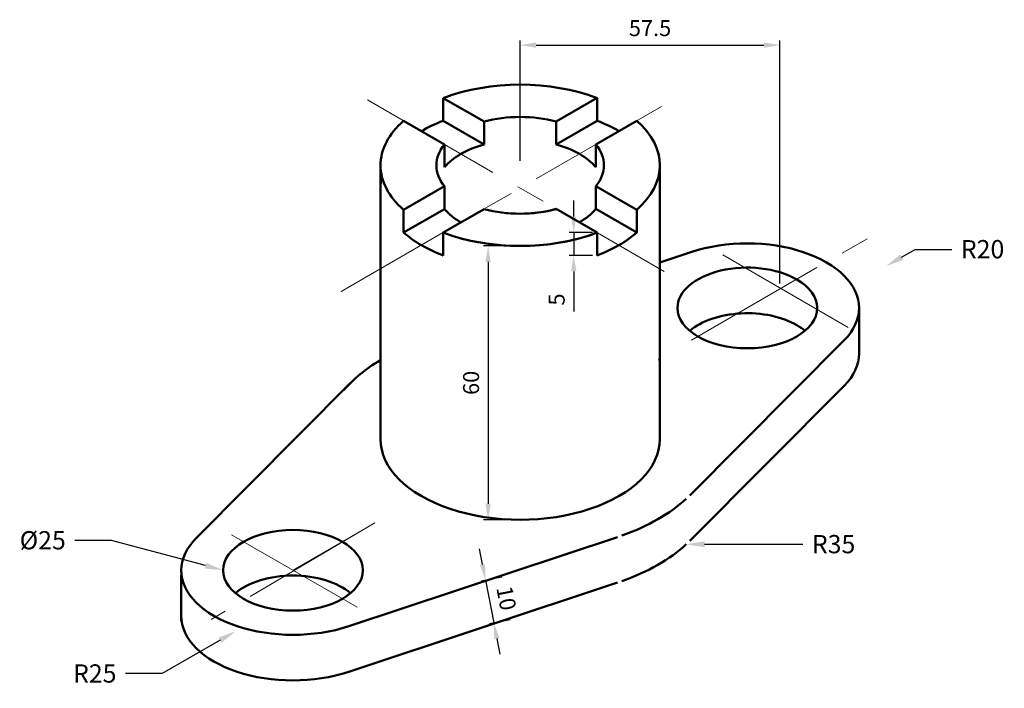
# Model space of a CAD drawing. Units: millimetres. Extents: x 2300 to 2516, y 894 to 1041.
import ezdxf
from ezdxf import colors
from ezdxf.entities.mleader import LeaderData, LeaderLine
from ezdxf.math import Vec2, Vec3

# ---------------------------------------------------------------- set-up
doc = ezdxf.new("R2010")
doc.units = ezdxf.units.MM
doc.linetypes.add('CENTER', pattern=[50.8, 31.75, -6.35, 6.35, -6.35])
for name, color, linetype, lineweight in [('M-CNTR', 1, 'CENTER', 18), ('M-DIMS', 3, 'Continuous', 25), ('M-OUTL', 7, 'Continuous', 50)]:
    doc.layers.add(name, color=color, linetype=linetype, lineweight=lineweight)
doc.styles.get("Standard").update_dxf_attribs({"font": 'arial.ttf'})
doc.dimstyles.new('AM_ISO$0', dxfattribs={"dimtxt": 3.5, "dimasz": 3.5, "dimexe": 1, "dimexo": 1, "dimgap": 1.5, "dimtad": 1, "dimdsep": 46, "dimtxsty": 'Standard', "dimcen": 0, "dimclrd": 256, "dimclre": 256, "dimclrt": 2, "dimadec": 0, "dimazin": 2, "dimtp": 0.1, "dimtm": 0.1, "dimtfac": 0.71, "dimtdec": 3, "dimtmove": 0, "dimatfit": 3, "dimfxl": 1, "dimlwd": -1, "dimlwe": -1, "dimarcsym": 1})

# ---------------------------------------------------------------- blocks, each defined once
blk = doc.blocks.new('*D3')
at = {"layer": 'Defpoints', "color": 0, "transparency": 16777216}
for p in [(2406.88, 918.66), (2408.7, 909.3), (2404.15, 908.42)]:
    blk.add_point(p, dxfattribs=at)
at = {"layer": 'M-DIMS', "color": 0, "linetype": 'ByBlock', "transparency": 16777216}
for p, q in [((2401.66, 921.21), (2400.99, 924.65)), ((2405.9, 918.47), (2401.34, 917.59)), ((2402.33, 917.78), (2404.15, 908.42)), ((2407.72, 909.11), (2403.17, 908.23)), ((2404.82, 904.98), (2405.48, 901.55))]:
    blk.add_line(p, q, dxfattribs=at)
at = {"layer": 'M-DIMS', "color": 0, "transparency": 16777216}
for points in [[(2402.23, 921.33), (2401.09, 921.1), (2402.33, 917.78)], [(2405.39, 905.09), (2404.24, 904.87), (2404.15, 908.42)]]:
    blk.add_solid(points, dxfattribs=at)
at = {"layer": 'M-DIMS', "color": 0, "transparency": 16777216, "insert": (2406.46, 913.73), "char_height": 3.5, "attachment_point": 5, "rotation": 281.0109}
blk.add_mtext('10', dxfattribs=at)
blk = doc.blocks.new('*D4')
at = {"layer": 'Defpoints', "color": 0, "transparency": 16777216}
for p in [(2409.91, 991.02), (2402.9, 931.02), (2409.91, 931.02)]:
    blk.add_point(p, dxfattribs=at)
at = {"layer": 'M-DIMS', "color": 0, "linetype": 'ByBlock', "transparency": 16777216}
for p, q in [((2408.91, 991.02), (2401.9, 991.02)), ((2402.9, 987.52), (2402.9, 934.52)), ((2408.91, 931.02), (2401.9, 931.02))]:
    blk.add_line(p, q, dxfattribs=at)
at = {"layer": 'M-DIMS', "color": 0, "transparency": 16777216}
for points in [[(2402.31, 987.52), (2403.48, 987.52), (2402.9, 991.02)], [(2402.31, 934.52), (2403.48, 934.52), (2402.9, 931.02)]]:
    blk.add_solid(points, dxfattribs=at)
at = {"layer": 'M-DIMS', "color": 0, "transparency": 16777216, "insert": (2399.61, 961.02), "char_height": 3.5, "attachment_point": 5, "rotation": 90}
blk.add_mtext('60', dxfattribs=at)
blk = doc.blocks.new('*D5')
at = {"layer": 'Defpoints', "color": 0, "transparency": 16777216}
for p in [(2466.86, 1035.03), (2409.91, 1008.7), (2466.86, 981.83)]:
    blk.add_point(p, dxfattribs=at)
at = {"layer": 'M-DIMS', "color": 0, "linetype": 'ByBlock', "transparency": 16777216}
for p, q in [((2409.91, 1009.7), (2409.91, 1036.03)), ((2466.86, 982.83), (2466.86, 1036.03)), ((2413.41, 1035.03), (2463.36, 1035.03))]:
    blk.add_line(p, q, dxfattribs=at)
at = {"layer": 'M-DIMS', "color": 0, "transparency": 16777216}
for points in [[(2413.41, 1035.62), (2413.41, 1034.45), (2409.91, 1035.03)], [(2463.36, 1035.62), (2463.36, 1034.45), (2466.86, 1035.03)]]:
    blk.add_solid(points, dxfattribs=at)
at = {"layer": 'M-DIMS', "color": 0, "transparency": 16777216, "insert": (2438.39, 1038.31), "char_height": 3.5, "attachment_point": 5}
blk.add_mtext('57.5', dxfattribs=at)
blk = doc.blocks.new('*D6')
at = {"layer": 'Defpoints', "color": 0, "transparency": 16777216}
for p in [(2426.8, 993.95), (2421.66, 988.95), (2426.8, 988.95)]:
    blk.add_point(p, dxfattribs=at)
at = {"layer": 'M-DIMS', "color": 0, "linetype": 'ByBlock', "transparency": 16777216}
for p, q in [((2421.66, 997.45), (2421.66, 1000.95)), ((2425.8, 993.95), (2420.66, 993.95)), ((2421.66, 993.95), (2421.66, 988.95)), ((2425.8, 988.95), (2420.66, 988.95)), ((2421.66, 985.45), (2421.66, 976.63))]:
    blk.add_line(p, q, dxfattribs=at)
at = {"layer": 'M-DIMS', "color": 0, "transparency": 16777216}
for points in [[(2421.07, 997.45), (2422.24, 997.45), (2421.66, 993.95)], [(2421.07, 985.45), (2422.24, 985.45), (2421.66, 988.95)]]:
    blk.add_solid(points, dxfattribs=at)
at = {"layer": 'M-DIMS', "color": 0, "transparency": 16777216, "insert": (2418.38, 979.29), "char_height": 3.5, "attachment_point": 5, "rotation": 90}
blk.add_mtext('5', dxfattribs=at)

msp = doc.modelspace()

# ---------------------------------------------------------------- linework, layer by layer
at = {"layer": 'M-CNTR'}
for p, q in [((2376.431, 1023.034), (2441.512, 985.46)), ((2440.919, 1021.602), (2370.647, 981.031)), ((2447.487, 970.395), (2486.858, 993.125)), ((2481.818, 973.189), (2451.899, 990.462)), ((2378.08, 930.322), (2342.182, 909.16)), ((2360.118, 919.952), (2378.08, 930.322)), ((2374.174, 911.837), (2345.195, 928.568))]:
    msp.add_line(p, q, dxfattribs=at)
at = {"layer": 'M-OUTL'}
for p, q in [((2393.039, 1018.442), (2393.039, 1023.442)), ((2402.005, 1018.265), (2393.039, 1023.442)), ((2426.798, 1023.45), (2417.832, 1018.273)), ((2426.798, 1023.45), (2426.798, 1018.45)), ((2393.344, 1013.265), (2384.379, 1018.442)), ((2402.005, 1013.265), (2393.039, 1018.442)), ((2402.005, 1013.265), (2402.005, 1018.265)), ((2417.832, 1018.273), (2417.832, 1013.273)), ((2417.839, 1013.265), (2426.805, 1018.442)), ((2435.458, 1018.45), (2426.492, 1013.273)), ((2393.344, 1008.265), (2393.344, 1013.265)), ((2426.492, 1013.273), (2426.492, 1008.273)), ((2379.296, 948.702), (2379.296, 1008.702)), ((2440.534, 1008.702), (2440.534, 948.702)), ((2384.379, 998.947), (2393.344, 1004.123)), ((2393.344, 999.123), (2393.344, 1004.123)), ((2435.458, 998.955), (2426.492, 1004.131)), ((2426.492, 1004.131), (2426.492, 999.131)), ((2384.379, 993.947), (2393.344, 999.123)), ((2384.379, 993.947), (2384.379, 998.947)), ((2393.039, 993.947), (2402.005, 999.123)), ((2417.832, 999.131), (2426.798, 993.955)), ((2435.458, 993.955), (2426.492, 999.131)), ((2435.458, 993.955), (2435.458, 998.955)), ((2393.039, 988.947), (2393.039, 993.947)), ((2426.798, 993.955), (2426.798, 988.955)), ((2440.541, 987.393), (2447.516, 989.707)), ((2484.213, 977.444), (2484.213, 967.444)), ((2480.958, 970.399), (2447.09, 936.366)), ((2338.886, 926.989), (2372.753, 961.023)), ((2480.958, 960.399), (2447.09, 926.366)), ((2431.276, 927.235), (2372.328, 907.682)), ((2335.624, 908.791), (2335.624, 918.791)), ((2431.276, 917.235), (2372.328, 897.682))]:
    msp.add_line(p, q, dxfattribs=at)
for centre, major_axis, start_param, end_param in [((2409.922, 1008.694), (30.619, 0), 0.9867561, 2.1548366), ((2409.922, 1008.694), (18.371, 0), 1.1252351, 2.0163576), ((2409.922, 1008.694), (30.619, 0), 2.5575524, 3.1415927), ((2409.922, 1003.694), (30.619, 0), 2.1548366, 2.3561945), ((2409.915, 1003.702), (-30.619, 0), 10.2101761, 10.411534), ((2409.915, 1008.702), (-30.619, 0), 2.5575524, 3.7256329), ((2409.922, 1008.694), (18.371, 0), 2.6960314, 3.1415927), ((2409.922, 1003.694), (18.371, 0), 2.0163576, 2.6960314), ((2409.915, 1003.702), (-18.371, 0), 9.8703392, 10.550013), ((2409.915, 1008.702), (-18.371, 0), 2.6960314, 3.5871539), ((2409.922, 1008.694), (30.619, 0), 3.1415927, 3.7256329), ((2409.922, 1008.694), (18.371, 0), 3.1415927, 3.5871539), ((2409.915, 1003.702), (-30.619, 0), 6.1412883, 6.2831853), ((2409.922, 1003.694), (18.371, 0), 3.5871539, 3.9269908), ((2409.922, 1008.694), (18.371, 0), 4.2668277, 5.1579502), ((2409.915, 1008.702), (-18.371, 0), 1.3884849, 2.0163576), ((2409.915, 1003.702), (-18.371, 0), 8.6393798, 8.9792167), ((2409.922, 1003.694), (30.619, 0), 3.7256329, 4.1283487), ((2409.922, 1008.694), (30.619, 0), 4.1283487, 5.2964292), ((2409.915, 1008.702), (-30.619, 0), 1.1326473, 2.1548366), ((2409.915, 1003.702), (-30.619, 0), 8.4380219, 8.8407377), ((2459.718, 977.444), (-24.495, 0), 3.1415927, 5.2338643), ((2459.718, 977.444), (15.309, 0), 0.7853982, 3.1415927), ((2459.718, 977.444), (15.309, 0), 0, 0.7853982), ((2459.718, 977.444), (15.309, 0), 3.1415927, 6.2831853), ((2459.718, 967.444), (15.309, 0), 0.7853982, 2.5403284), ((2459.718, 977.444), (-24.495, 0), 2.6201174, 3.1415927), ((2459.718, 967.444), (15.309, 0), 0.6012642, 0.7853982), ((2459.718, 967.444), (-24.495, 0), 2.6201174, 3.1415927), ((2409.915, 948.702), (-42.866, 0), 5.5079919, 5.835769), ((2409.915, 948.702), (-42.866, 0), 10.1999713, 10.2101761), ((2409.915, 948.702), (-30.619, 0), 6.2831853, 9.424778), ((2409.915, 948.702), (-42.866, 0), 8.4006285, 8.868858), ((2360.125, 919.944), (-24.495, 0), 5.76171, 6.2831853), ((2409.915, 938.702), (-42.866, 0), 8.4006285, 8.868858), ((2360.125, 919.944), (-24.495, 0), 0, 2.0922716), ((2360.118, 909.952), (-15.309, 0), 3.7428569, 5.6819211), ((2360.125, 909.944), (-24.495, 0), 0, 2.0922716)]:
    msp.add_ellipse(centre, major_axis=major_axis, ratio=0.5773503, start_param=start_param, end_param=end_param, dxfattribs=at)
msp.add_ellipse((2360.118, 919.952), major_axis=(-15.309, 0), ratio=0.5773503, dxfattribs=at)

# ---------------------------------------------------------------- dimensions: what is measured, and where the dimension line sits
at = {"layer": 'M-DIMS'}
dim = msp.add_linear_dim(base=(2466.859, 1035.034), p1=(2409.915, 1008.702), p2=(2466.859, 981.826), text='57.5', dimstyle='AM_ISO$0', override={"dimpost": '', "dimclrd": 0, "dimclre": 0, "dimclrt": 0}, dxfattribs=at)
dim.commit()
dim.dimension.update_dxf_attribs({"geometry": '*D5', "text_midpoint": (2438.387, 1038.314)})
dim = msp.add_linear_dim(base=(2421.655, 988.955), p1=(2426.798, 993.955), p2=(2426.798, 988.955), angle=90, dimstyle='AM_ISO$0', override={"dimclrd": 0, "dimclre": 0, "dimclrt": 0}, dxfattribs=at)
dim.commit()
dim.dimension.update_dxf_attribs({"geometry": '*D6', "text_midpoint": (2421.655, 979.294), "dimtype": 160})
dim = msp.add_aligned_dim(p1=(2409.915, 991.024), p2=(2409.915, 931.024), distance=-7.02, dimstyle='AM_ISO$0', override={"dimpost": '', "dimclrd": 0, "dimclre": 0, "dimclrt": 0}, dxfattribs=at)
dim.commit()
dim.dimension.update_dxf_attribs({"geometry": '*D4', "text_midpoint": (2399.608, 961.024)})
dim = msp.add_aligned_dim(p1=(2406.877, 918.664), p2=(2408.698, 909.304), distance=-4.636, text='10', dimstyle='AM_ISO$0', override={"dimpost": '', "dimclrd": 0, "dimclre": 0, "dimclrt": 0}, dxfattribs=at)
dim.commit()
dim.dimension.update_dxf_attribs({"geometry": '*D3', "text_midpoint": (2406.464, 913.727)})

# ---------------------------------------------------------------- leaders
ml = msp.add_multileader_mtext('Standard', dxfattribs=at)
ml.set_content('{\\C2;R20}', color=256)
ml.set_leader_properties()
ml.build(insert=Vec2(0, 0))
ctx = ml.context
ctx.base_point, ctx.plane_origin = Vec3(2504.521, 990.283), Vec3(2490.076, 986.561)
notes = []
notes.append((ctx, [(0, (1, 1, 0), (2496.521, 990.283), (1, 0), 8, [(0, [(2490.076, 986.561)], 0, [])])]))
ctx.mtext.insert, ctx.mtext.flow_direction = Vec3(2506.521, 992.317), 5
ml = msp.add_multileader_mtext('Standard', dxfattribs=at)
ml.set_content('{\\C2;%%C25}', color=256)
ml.set_leader_properties()
ml.build(insert=Vec2(0, 0))
ctx = ml.context
ctx.base_point, ctx.plane_origin = Vec3(2298.21, 926.449), Vec3(2344.809, 919.952)
ctx.text_align_type = 2
notes.append((ctx, [(0, (1, 1, 0), (2320.322, 926.449), (-1, 0), 8, [(0, [(2344.809, 919.952)], 0, [])])]))
ctx.mtext.insert, ctx.mtext.alignment, ctx.mtext.flow_direction = Vec3(2310.322, 928.529), 3, 5
ml = msp.add_multileader_mtext('Standard', dxfattribs=at)
ml.set_content('{\\C2;R35}', color=256)
ml.set_leader_properties()
ml.build(insert=Vec2(0, 0))
ctx = ml.context
ctx.base_point, ctx.plane_origin = Vec3(2471.861, 925.642), Vec3(2446.326, 925.642)
notes.append((ctx, [(0, (1, 1, 0), (2463.861, 925.642), (1, 0), 8, [(0, [(2446.326, 925.642)], 0, [])])]))
ctx.mtext.insert, ctx.mtext.flow_direction = Vec3(2473.861, 927.677), 5
ml = msp.add_multileader_mtext('Standard', dxfattribs=at)
ml.set_content('{\\C2;R25}', color=256)
ml.set_leader_properties()
ml.build(insert=Vec2(0, 0))
ctx = ml.context
ctx.base_point, ctx.plane_origin = Vec3(2309.846, 897.297), Vec3(2347.605, 906.634)
ctx.text_align_type = 2
notes.append((ctx, [(0, (1, 1, 0), (2331.434, 897.297), (-1, 0), 8, [(0, [(2347.605, 906.634)], 0, [])])]))
ctx.mtext.insert, ctx.mtext.alignment, ctx.mtext.flow_direction = Vec3(2321.434, 899.331), 3, 5
for ctx, leaders in notes:
    for number, flags, end, landing, length, lines in leaders:
        leader = LeaderData()
        leader.index, (leader.has_last_leader_line, leader.has_dogleg_vector, leader.attachment_direction) = number, flags
        leader.last_leader_point, leader.dogleg_vector, leader.dogleg_length = Vec3(end), Vec3(landing), length
        for number, points, colour, breaks in lines:
            line = LeaderLine()
            line.index, line.vertices, line.color, line.breaks = number, Vec3.list(points), colors.encode_raw_color(colour), breaks
            leader.lines.append(line)
        ctx.leaders.append(leader)

doc.saveas('drawing.dxf')
